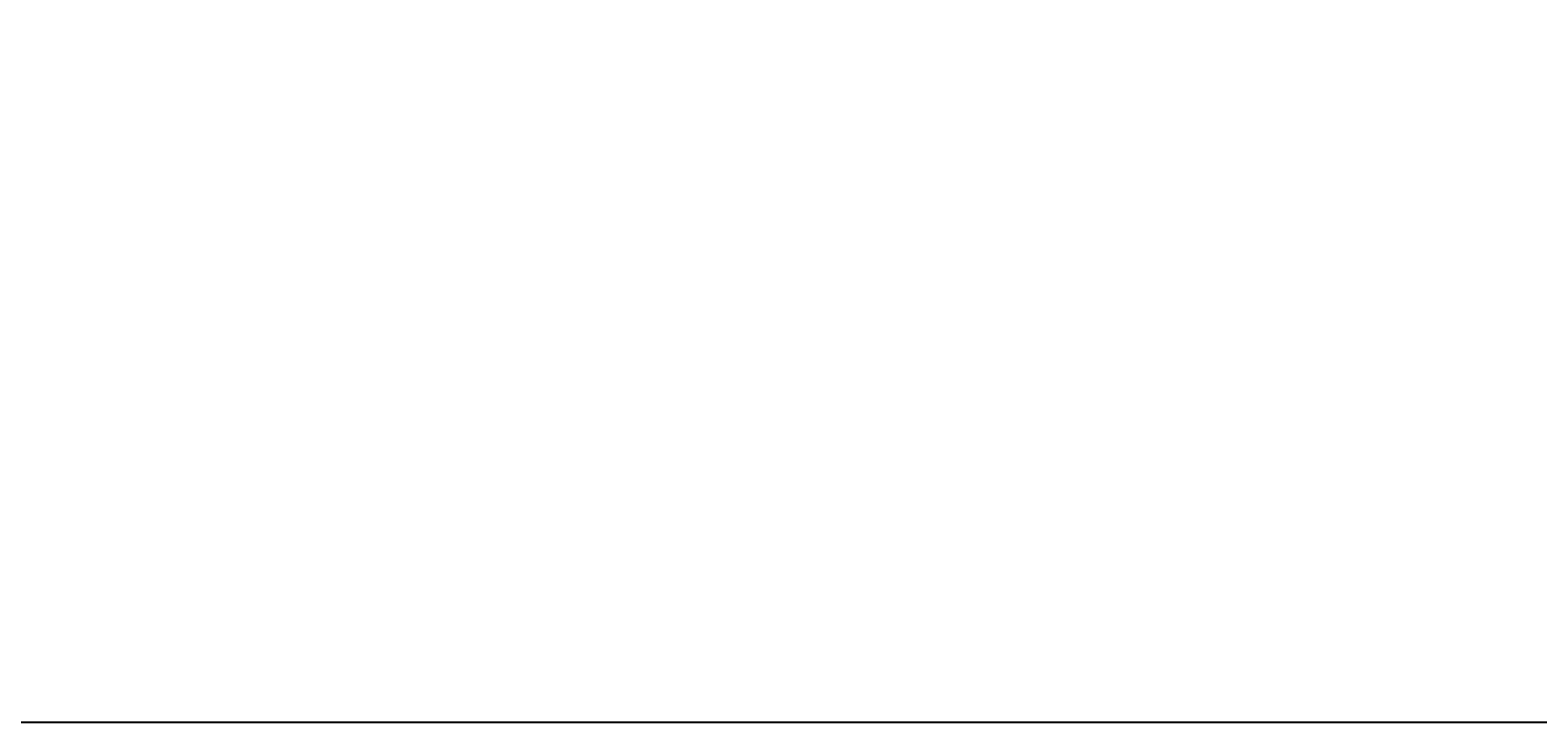
# Model space of a CAD drawing. Units: inches. Extents: x -61 to 1599, y -1316 to 257.
# Tile 2 of 204: x 99 to 259, y -1316 to -1242. Entities that reach past the tile are written whole.
import ezdxf

# ---------------------------------------------------------------- set-up
doc = ezdxf.new("R2010")
doc.units = ezdxf.units.IN
doc.header["$MEASUREMENT"] = 0
doc.layers.add('A-ANNO-DIMS', color=2, linetype='Continuous', lineweight=18)
doc.styles.get("Standard").update_dxf_attribs({"font": 'arial.ttf'})
doc.dimstyles.get("Standard").update_dxf_attribs({"dimtxt": 0.18, "dimasz": 0.18, "dimexe": 0.18, "dimexo": 0.0625, "dimgap": 0.09, "dimtad": 0, "dimtih": 1, "dimtoh": 1, "dimdec": 0, "dimzin": 0, "dimdsep": 46, "dimlunit": 3, "dimtxsty": 'Standard', "dimcen": 0.09, "dimadec": 0, "dimazin": 0, "dimtfac": 1, "dimtdec": 0, "dimtofl": 0, "dimtmove": 0, "dimatfit": 3, "dimfxl": 1, "dimtolj": 1, "dimtzin": 0, "dimarcsym": 0})

# ---------------------------------------------------------------- blocks, each defined once
blk = doc.blocks.new('*D688')
at = {"layer": 'A-ANNO-DIMS', "color": 0, "lineweight": -2, "transparency": 16777216}
for p, q in [((14.7, -1216.01), (14.7, -1315.72)), ((544.7, -1216.01), (544.7, -1315.72)), ((14.88, -1315.54), (279.41, -1315.54)), ((544.52, -1315.54), (279.99, -1315.54))]:
    blk.add_line(p, q, dxfattribs=at)
at = {"layer": 'A-ANNO-DIMS', "color": 0, "transparency": 16777216}
for points in [[(14.88, -1315.51), (14.88, -1315.57), (14.7, -1315.54)], [(544.52, -1315.51), (544.52, -1315.57), (544.7, -1315.54)]]:
    blk.add_solid(points, dxfattribs=at)
at = {"layer": 'DEFPOINTS', "color": 0, "transparency": 16777216}
for p in [(14.7, -1215.94), (544.7, -1215.94), (544.7, -1315.54)]:
    blk.add_point(p, dxfattribs=at)
at = {"layer": 'A-ANNO-DIMS', "color": 0, "transparency": 16777216, "insert": (279.7, -1315.54), "char_height": 0.18, "attachment_point": 5}
blk.add_mtext('\\A1;530', dxfattribs=at)

msp = doc.modelspace()

# ---------------------------------------------------------------- dimensions: what is measured, and where the dimension line sits
at = {"layer": 'A-ANNO-DIMS'}
dim = msp.add_linear_dim(base=(544.7028, -1315.5446), p1=(14.7028, -1215.9446), p2=(544.7028, -1215.9446), dimstyle='Standard', override={"dimdec": 0, "dimlfac": 1, "dimrnd": 0, "dimzin": 0, "dimdsep": 46, "dimlunit": 2}, dxfattribs=at)
dim.commit()
dim.dimension.update_dxf_attribs({"geometry": '*D688', "text_midpoint": (279.7028, -1315.5446)})

doc.saveas('drawing.dxf')
